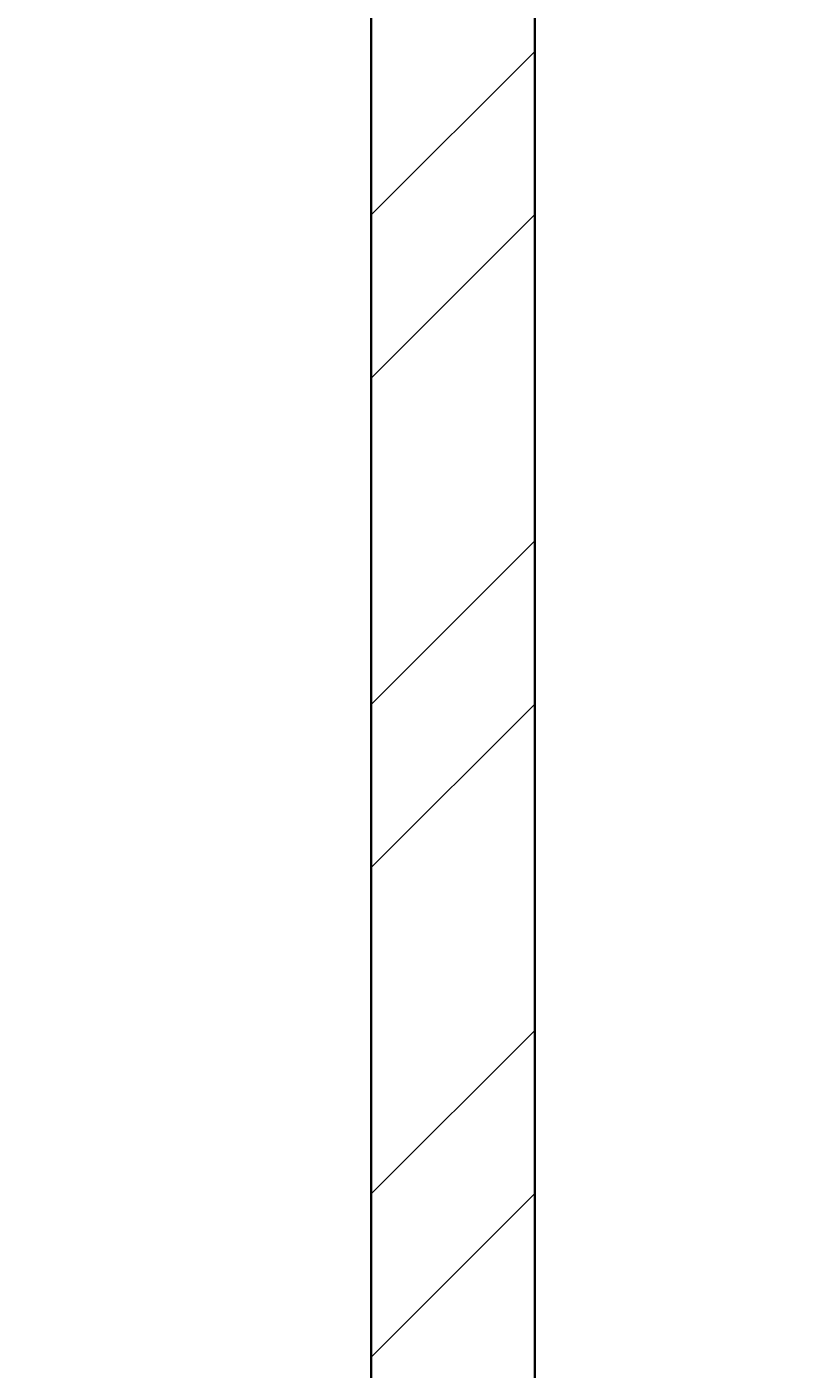
# Model space of a CAD drawing. Units: inches. Extents: x 1962 to 2771, y 1245 to 2660.
# Tile 54 of 114: x 2225 to 2247, y 2068 to 2105. Entities that reach past the tile are written whole.
import ezdxf

# ---------------------------------------------------------------- set-up
doc = ezdxf.new("R2010")
doc.units = ezdxf.units.IN
for name, color, linetype, lineweight in [('A-ANNO-DIMS', 2, 'Continuous', 18), ('A-WALL', 7, 'Continuous', 35), ('A-WALL-PATT', 252, 'Continuous', 13)]:
    doc.layers.add(name, color=color, linetype=linetype, lineweight=lineweight)
doc.styles.get("Standard").update_dxf_attribs({"font": 'arial.ttf'})
doc.dimstyles.get("Standard").update_dxf_attribs({"dimtxt": 0.18, "dimasz": 0.18, "dimexe": 0.18, "dimexo": 0.0625, "dimgap": 0.09, "dimtad": 0, "dimtih": 1, "dimtoh": 1, "dimdec": 4, "dimzin": 0, "dimdsep": 46, "dimtxsty": 'Standard', "dimcen": 0.09, "dimadec": 0, "dimazin": 0, "dimtfac": 1, "dimtdec": 4, "dimtofl": 0, "dimtmove": 0, "dimatfit": 3, "dimfxl": 1, "dimtolj": 1, "dimtzin": 0, "dimarcsym": 0})

# ---------------------------------------------------------------- blocks, each defined once
blk = doc.blocks.new('*D40')
at = {"layer": 'A-ANNO-DIMS', "color": 0, "lineweight": -2, "transparency": 16777216}
for p, q in [((2072.02, 2033.906), (2072.02, 2583.474)), ((2072.2, 2583.294), (2366.02, 2583.294)), ((2660.627, 2583.294), (2366.808, 2583.294)), ((2660.807, 2524.406), (2660.807, 2583.474))]:
    blk.add_line(p, q, dxfattribs=at)
at = {"layer": 'A-ANNO-DIMS', "color": 0, "transparency": 16777216}
for points in [[(2072.2, 2583.324), (2072.2, 2583.264), (2072.02, 2583.294)], [(2660.627, 2583.324), (2660.627, 2583.264), (2660.807, 2583.294)]]:
    blk.add_solid(points, dxfattribs=at)
at = {"layer": 'Defpoints', "color": 0, "transparency": 16777216}
for p in [(2660.807, 2583.294), (2660.807, 2524.344), (2072.02, 2033.844)]:
    blk.add_point(p, dxfattribs=at)
at = {"layer": 'A-ANNO-DIMS', "color": 0, "transparency": 16777216, "insert": (2366.414, 2583.294), "char_height": 0.18, "attachment_point": 5}
blk.add_mtext('\\A1;588.8', dxfattribs=at)

msp = doc.modelspace()

# ---------------------------------------------------------------- hatches: boundary and pattern name
at = {"layer": 'A-WALL-PATT'}
h = msp.add_hatch(dxfattribs=at)
h.set_pattern_fill('ANSI32', color=256)
h.paths.add_polyline_path([(2090.8074, 2467.3437), (2141.6481, 2467.3437), (2141.6481, 2469.5937), (2141.6481, 2471.8437), (2086.3074, 2471.8437), (2086.3074, 2422.5333), (2090.8074, 2422.5333)])
h.paths.add_polyline_path([(2282.7664, 2471.8437), (2204.8982, 2471.8437), (2204.8982, 2467.3437), (2234.8074, 2467.3437), (2234.8074, 2311.3437), (2228.7492, 2311.3437), (2228.7492, 2306.8437), (2234.8074, 2306.8437), (2331.9227, 2306.8437), (2331.9227, 2309.0937), (2331.9227, 2311.3437), (2239.3074, 2311.3437), (2239.3074, 2467.3437), (2282.7664, 2467.3437), (2282.7664, 2469.5937)])
h.paths.add_polyline_path([(2471.4531, 2519.8437), (2552.011, 2519.8437), (2564.3996, 2519.8437), (2564.3996, 2511.1389), (2568.8996, 2511.1389), (2568.8996, 2524.3437), (2466.9531, 2524.3437), (2466.9531, 2471.8437), (2450.0749, 2471.8437), (2446.4672, 2471.8437), (2446.4672, 2467.3437), (2450.0749, 2467.3437), (2475.9988, 2467.3437), (2475.9988, 2469.5937), (2475.9988, 2471.8437), (2471.4531, 2471.8437)])
h.paths.add_polyline_path([(2575.2231, 2469.5937), (2575.2231, 2471.8437), (2568.8996, 2471.8437), (2568.8996, 2487.1389), (2564.3996, 2487.1389), (2564.3996, 2471.8437), (2556.511, 2471.8437), (2499.2904, 2471.8437), (2499.2904, 2467.3437), (2507.8074, 2467.3437), (2507.8074, 2311.3437), (2414.863, 2311.3437), (2414.863, 2306.8437), (2512.3074, 2306.8437), (2517.0114, 2306.8437), (2517.0114, 2309.0937), (2517.0114, 2311.3437), (2512.3074, 2311.3437), (2512.3074, 2467.3437), (2575.2231, 2467.3437)])
h.paths.add_polyline_path([(2660.8074, 2471.8437), (2600.9602, 2471.8437), (2600.9602, 2467.3437), (2656.3074, 2467.3437), (2656.3074, 2432.5704), (2660.8074, 2432.5704)])
h.paths.add_polyline_path([(2660.8074, 2372.5704), (2656.3074, 2372.5704), (2656.3074, 2311.3437), (2600.276, 2311.3437), (2600.276, 2309.0937), (2600.276, 2306.8437), (2656.3074, 2306.8437), (2656.3074, 2296.2593), (2660.8074, 2296.2593)])
h.paths.add_polyline_path([(2572.3074, 2306.8437), (2577.1385, 2306.8437), (2577.1385, 2311.3437), (2551.082, 2311.3437), (2551.082, 2306.8437), (2567.8074, 2306.8437), (2567.8074, 2258.8437), (2540.0574, 2258.8437), (2540.0574, 2256.5937), (2540.0574, 2254.3437), (2567.8074, 2254.3437), (2656.3074, 2254.3437), (2656.3074, 2236.9085), (2660.8074, 2236.9085), (2660.8074, 2272.2593), (2656.3074, 2272.2593), (2656.3074, 2258.8437), (2572.3074, 2258.8437)])
h.paths.add_polyline_path([(2512.3074, 2254.3437), (2518.8716, 2254.3437), (2518.8716, 2256.5937), (2518.8716, 2258.8437), (2507.8074, 2258.8437), (2507.8074, 2177.8437), (2567.8074, 2177.8437), (2567.8074, 2172.9628), (2572.3074, 2172.9628), (2572.3074, 2177.8437), (2656.3074, 2177.8437), (2656.3074, 2166.4846), (2660.8074, 2166.4846), (2660.8074, 2200.9085), (2656.3074, 2200.9085), (2656.3074, 2182.3437), (2512.3074, 2182.3437)])
h.paths.add_polyline_path([(2656.3074, 2129.8437), (2572.3074, 2129.8437), (2572.3074, 2150.3044), (2570.0574, 2150.3044), (2567.8074, 2150.3044), (2567.8074, 2129.8437), (2507.8074, 2129.8437), (2507.8074, 2116.3027), (2510.0574, 2116.3027), (2512.3074, 2116.3027), (2512.3074, 2125.3437), (2567.8074, 2125.3437), (2572.3074, 2125.3437), (2656.3074, 2125.3437)])
h.paths.add_polyline_path([(2090.8074, 2362.5333), (2086.3074, 2362.5333), (2086.3074, 2298.6242), (2090.8074, 2298.6242), (2090.8074, 2306.8437), (2174.8074, 2306.8437), (2174.8074, 2286.4178), (2179.3074, 2286.4178), (2179.3074, 2306.8437), (2192.8641, 2306.8437), (2192.8641, 2309.0937), (2192.8641, 2311.3437), (2090.8074, 2311.3437)])
h.paths.add_polyline_path([(2209.156, 2258.8437), (2179.3074, 2258.8437), (2179.3074, 2263.2236), (2177.0574, 2263.2236), (2174.8074, 2263.2236), (2174.8074, 2258.8437), (2090.8074, 2258.8437), (2090.8074, 2274.6242), (2086.3074, 2274.6242), (2086.3074, 2238.2967), (2088.5574, 2238.2967), (2090.8074, 2238.2967), (2090.8074, 2254.3437), (2209.156, 2254.3437)])
h.paths.add_polyline_path([(2090.8074, 2177.8437), (2234.8074, 2177.8437), (2234.8074, 2173.1428), (2239.3074, 2173.1428), (2239.3074, 2258.8437), (2230.8442, 2258.8437), (2230.8442, 2256.5937), (2230.8442, 2254.3437), (2234.8074, 2254.3437), (2234.8074, 2182.3437), (2090.8074, 2182.3437), (2090.8074, 2202.2967), (2086.3074, 2202.2967), (2086.3074, 2140.0389), (2090.8074, 2140.0389)])
h.paths.add_polyline_path([(2090.8074, 2080.0389), (2086.3074, 2080.0389), (2086.3074, 2033.8437), (2090.8074, 2033.8437)], flags=17)
h.paths.add_polyline_path([(2244.9405, 2033.8437), (2239.3074, 2033.8437), (2239.3074, 2142.0665), (2237.2592, 2142.0665), (2234.8074, 2142.0665), (2234.8074, 2033.8437), (2090.8074, 2033.8437), (2076.5204, 2033.8437), (2072.0204, 2033.8437), (2072.0204, 2000.4493), (2076.5204, 2000.4493), (2076.5204, 2029.3437), (2090.8074, 2029.3437), (2244.9405, 2029.3437), (2244.9405, 2031.5937)])
h.paths.add_polyline_path([(2234.8074, 1933.3437), (2076.5204, 1933.3437), (2076.5204, 1952.4493), (2074.2704, 1952.4493), (2072.0204, 1952.4493), (2072.0204, 1933.3437), (2072.0204, 1928.8437), (2234.8074, 1928.8437)])
h.paths.add_polyline_path([(2090.8074, 1928.8437), (2086.3074, 1928.8437), (2086.3074, 1906.5013), (2090.8074, 1906.5013)])
h.paths.add_polyline_path([(2090.8074, 1846.5013), (2086.3074, 1846.5013), (2086.3074, 1769.9917), (2088.5574, 1769.9917), (2090.8074, 1769.9917), (2090.8074, 1780.3437), (2234.8074, 1780.3437), (2234.8074, 1708.3437), (2230.3764, 1708.3437), (2230.3764, 1703.8437), (2239.3074, 1703.8437), (2239.3074, 1792.6669), (2237.0574, 1792.6669), (2234.8074, 1792.6669), (2234.8074, 1784.8437), (2090.8074, 1784.8437)])
h.paths.add_polyline_path([(2239.3074, 1928.8437), (2244.9405, 1928.8437), (2244.9405, 1931.0937), (2244.9405, 1933.3437), (2234.8074, 1933.3437), (2234.8074, 1928.8437), (2234.8074, 1825.5949), (2239.3074, 1825.5949)])
h.paths.add_polyline_path([(2148.0425, 1649.0937), (2148.0425, 1651.3437), (2090.8074, 1651.3437), (2090.8074, 1646.8437), (2148.0425, 1646.8437)], flags=0)
h.paths.add_polyline_path([(2207.5601, 1708.3437), (2090.8074, 1708.3437), (2090.8074, 1703.8437), (2174.8074, 1703.8437), (2174.8074, 1651.3437), (2170.4457, 1651.3437), (2170.4457, 1646.8437), (2195.9924, 1646.8437), (2195.9924, 1649.0937), (2195.9924, 1651.3437), (2179.3074, 1651.3437), (2179.3074, 1703.8437), (2207.5601, 1703.8437), (2207.5601, 1706.0937)])
h.paths.add_polyline_path([(2090.8074, 1733.9917), (2086.3074, 1733.9917), (2086.3074, 1696.1032), (2088.5574, 1696.1032), (2090.8074, 1696.1032)])
h.paths.add_polyline_path([(2090.8074, 1672.1032), (2086.3074, 1672.1032), (2086.3074, 1600.3335), (2090.8074, 1600.3335)])
h.paths.add_polyline_path([(2090.8074, 1540.3335), (2086.3074, 1540.3335), (2086.3074, 1486.3437), (2139.6766, 1486.3437), (2139.6766, 1490.8437), (2090.8074, 1490.8437)])
h.paths.add_polyline_path([(2302.3876, 1490.8437), (2239.3074, 1490.8437), (2239.3074, 1646.8437), (2335.9994, 1646.8437), (2335.9994, 1651.3437), (2229.884, 1651.3437), (2229.884, 1646.8437), (2234.8074, 1646.8437), (2234.8074, 1490.8437), (2202.7103, 1490.8437), (2202.7103, 1488.5937), (2202.7103, 1486.3437), (2275.0699, 1486.3437), (2275.0699, 1475.772), (2279.5699, 1475.772), (2279.5699, 1486.3437), (2302.3876, 1486.3437)])
h.paths.add_polyline_path([(2279.5699, 1451.772), (2275.0699, 1451.772), (2275.0699, 1438.3437), (2174.8074, 1438.3437), (2174.8074, 1486.3437), (2179.7922, 1486.3437), (2179.7922, 1490.8437), (2163.3585, 1490.8437), (2163.3585, 1488.5937), (2163.3585, 1486.3437), (2170.3074, 1486.3437), (2170.3074, 1433.8437), (2279.5699, 1433.8437)])
h.paths.add_polyline_path([(2427.2363, 1490.8437), (2375.8074, 1490.8437), (2375.8074, 1646.8437), (2381.6401, 1646.8437), (2381.6401, 1651.3437), (2365.887, 1651.3437), (2365.887, 1649.0937), (2365.887, 1646.8437), (2371.3074, 1646.8437), (2371.3074, 1490.8437), (2327.5627, 1490.8437), (2327.5627, 1488.5937), (2327.5627, 1486.3437), (2371.3074, 1486.3437), (2371.3074, 1433.8437), (2375.8074, 1433.8437), (2375.8074, 1486.3437), (2427.2363, 1486.3437)])
h.paths.add_polyline_path([(2512.3074, 1646.8437), (2519.4351, 1646.8437), (2519.4351, 1649.0937), (2519.4351, 1651.3437), (2507.8074, 1651.3437), (2416.0063, 1651.3437), (2416.0063, 1649.0937), (2416.0063, 1646.8437), (2507.8074, 1646.8437), (2507.8074, 1490.8437), (2497.0532, 1490.8437), (2497.0532, 1488.5937), (2497.0532, 1486.3437), (2574.9344, 1486.3437), (2574.9344, 1476.0181), (2579.4344, 1476.0181), (2579.4344, 1486.3437), (2584.4872, 1486.3437), (2584.3074, 1490.8437), (2512.3074, 1490.8437)])
h.paths.add_polyline_path([(2470.5091, 1486.3437), (2473.9767, 1486.3437), (2473.9767, 1490.8437), (2449.6605, 1490.8437), (2449.6605, 1488.5937), (2449.6605, 1486.3437), (2466.0091, 1486.3437), (2466.0091, 1433.8437), (2470.5091, 1433.8437), (2579.4344, 1433.8437), (2579.4344, 1452.0181), (2574.9344, 1452.0181), (2574.9344, 1438.3437), (2554.5091, 1438.3437), (2470.5091, 1438.3437)])
h.paths.add_polyline_path([(2656.3074, 1490.8437), (2611.86, 1490.8437), (2611.86, 1486.3437), (2656.3074, 1486.3437)])
h.paths.add_polyline_path([(2660.8074, 1532.7007), (2658.5574, 1532.7007), (2656.3074, 1532.7007), (2656.3074, 1486.3437), (2660.8074, 1486.3437)])
h.paths.add_polyline_path([(2660.8074, 1664.9663), (2656.3074, 1664.9663), (2656.3074, 1651.3437), (2602.2313, 1651.3437), (2602.2313, 1646.8437), (2656.3074, 1646.8437), (2656.3074, 1592.7007), (2660.8074, 1592.7007)])
h.paths.add_polyline_path([(2660.8074, 1724.5221), (2656.3074, 1724.5221), (2656.3074, 1703.8437), (2542.4725, 1703.8437), (2542.4725, 1699.3437), (2567.8074, 1699.3437), (2567.8074, 1651.3437), (2552.7766, 1651.3437), (2552.7766, 1649.0937), (2552.7766, 1646.8437), (2577.2878, 1646.8437), (2577.2878, 1649.0937), (2577.2878, 1651.3437), (2572.3074, 1651.3437), (2572.3074, 1699.3437), (2656.3074, 1699.3437), (2656.3074, 1688.9663), (2660.8074, 1688.9663)])
h.paths.add_polyline_path([(2660.8074, 1880.6524), (2656.3074, 1880.6524), (2656.3074, 1832.8437), (2512.3074, 1832.8437), (2512.3074, 1837.8959), (2507.8074, 1837.8959), (2507.8074, 1828.3437), (2567.8074, 1828.3437), (2567.8074, 1804.3437), (2572.3074, 1804.3437), (2572.3074, 1828.3437), (2656.3074, 1828.3437), (2656.3074, 1818.6778), (2660.8074, 1818.6778)])
h.paths.add_polyline_path([(2660.8074, 1794.6778), (2656.3074, 1794.6778), (2656.3074, 1780.3437), (2572.3074, 1780.3437), (2572.3074, 1783.0303), (2570.0574, 1783.0303), (2567.8074, 1783.0303), (2567.8074, 1780.3437), (2507.8074, 1780.3437), (2507.8074, 1699.3437), (2517.8858, 1699.3437), (2517.8858, 1701.5937), (2517.8858, 1703.8437), (2512.3074, 1703.8437), (2512.3074, 1775.8437), (2656.3074, 1775.8437), (2656.3074, 1760.5221), (2660.8074, 1760.5221)])
h.paths.add_polyline_path([(2660.8074, 1981.3437), (2660.8074, 2020.2808), (2658.5574, 2020.2808), (2656.3074, 2020.2808), (2656.3074, 1981.3437), (2512.3074, 1981.3437), (2512.3074, 2086.6996), (2507.8074, 2086.6996), (2507.8074, 1981.3437), (2375.8074, 1981.3437), (2375.8074, 1986.8505), (2373.5574, 1986.8505), (2371.3074, 1986.8505), (2371.3074, 1973.2607), (2375.8074, 1973.2607), (2375.8074, 1976.8437), (2507.8074, 1976.8437), (2507.8074, 1865.4281), (2510.0574, 1865.4281), (2512.3074, 1865.4281), (2512.3074, 1976.8437), (2660.8074, 1976.8437)])
h.paths.add_polyline_path([(2375.8074, 1940.297), (2373.5574, 1940.297), (2371.3074, 1940.297), (2371.3074, 1933.3437), (2278.4434, 1933.3437), (2278.4434, 1928.8437), (2371.3074, 1928.8437), (2371.3074, 1651.3437), (2375.8074, 1651.3437)])
h.paths.add_polyline_path([(2660.8074, 1976.8437), (2656.3074, 1976.8437), (2656.3074, 1940.6524), (2660.8074, 1940.6524)], flags=17)
h.paths.add_polyline_path([(2660.8074, 2142.4846), (2656.3074, 2142.4846), (2656.3074, 2080.2808), (2660.8074, 2080.2808)])
h.paths.add_polyline_path([(2381.4189, 2311.3437), (2375.8074, 2311.3437), (2375.8074, 2467.3437), (2424.7242, 2467.3437), (2424.7242, 2469.5937), (2424.7242, 2471.8437), (2375.8074, 2471.8437), (2375.8074, 2524.3437), (2371.3074, 2524.3437), (2371.3074, 2471.8437), (2307.2097, 2471.8437), (2307.2097, 2467.3437), (2371.3074, 2467.3437), (2371.3074, 2311.3437), (2366.8901, 2311.3437), (2366.8901, 2306.8437), (2371.3074, 2306.8437), (2371.3074, 2033.8437), (2279.6589, 2033.8437), (2279.6589, 2029.3437), (2371.3074, 2029.3437), (2371.3074, 2014.2598), (2375.8074, 2014.2598), (2375.8074, 2306.8437), (2381.4189, 2306.8437)])
h.paths.add_polyline_path([(2263.3074, 2524.3437), (2170.3074, 2524.3437), (2170.3074, 2519.8437), (2170.3074, 2471.8437), (2165.0312, 2471.8437), (2165.0312, 2467.3437), (2179.6721, 2467.3437), (2179.6721, 2469.5161), (2179.6721, 2471.8437), (2174.8074, 2471.8437), (2174.8074, 2519.8437), (2258.8074, 2519.8437), (2258.8074, 2511.6436), (2263.3074, 2511.6436)])
h.paths.add_polyline_path([(2245.0232, 1361.4123), (2492.9468, 1361.4123), (2492.9468, 1398.505), (2245.0232, 1398.505)], flags=9)
h.paths.add_polyline_path([(2388.1434, 2086.6936), (2425.0704, 2086.6936), (2425.0704, 2105.3509), (2388.1434, 2105.3509)], flags=9)
h.paths.add_polyline_path([(2404.922, 2242.6744), (2445.7337, 2242.6744), (2445.7337, 2261.3318), (2404.922, 2261.3318)], flags=9)
h.paths.add_polyline_path([(2269.4107, 2156.7935), (2306.3378, 2156.7935), (2306.3378, 2175.4508), (2269.4107, 2175.4508)], flags=9)
h.paths.add_polyline_path([(2269.3277, 2233.4343), (2306.2547, 2233.4343), (2306.2547, 2252.0917), (2269.3277, 2252.0917)], flags=9)
h.paths.add_polyline_path([(2431.6052, 2320.6922), (2470.4456, 2320.6922), (2470.4456, 2339.3495), (2431.6052, 2339.3495)], flags=25)
h.paths.add_polyline_path([(2249.6902, 2315.7608), (2288.5306, 2315.7608), (2288.5306, 2334.4182), (2249.6902, 2334.4182)], flags=25)
h.paths.add_polyline_path([(2096.9301, 2314.3181), (2135.7704, 2314.3181), (2135.7704, 2332.9755), (2096.9301, 2332.9755)], flags=25)
h.paths.add_polyline_path([(2134.3475, 2285.7089), (2161.4655, 2285.7089), (2161.4655, 2304.3662), (2134.3475, 2304.3662)], flags=9)
h.paths.add_polyline_path([(2126.5155, 2209.4076), (2159.9227, 2209.4076), (2159.9227, 2228.065), (2126.5155, 2228.065)], flags=25)
h.paths.add_polyline_path([(2110.5753, 2141.5299), (2149.4157, 2141.5299), (2149.4157, 2160.1872), (2110.5753, 2160.1872)], flags=25)
h.paths.add_polyline_path([(2249.8618, 1968.3317), (2286.3966, 1968.3317), (2286.3966, 1986.989), (2249.8618, 1986.989)], flags=9)
h.paths.add_polyline_path([(2395.9507, 1777.0051), (2436.7624, 1777.0051), (2436.7624, 1795.6625), (2395.9507, 1795.6625)], flags=9)
h.paths.add_polyline_path([(2398.5259, 1888.5651), (2435.0062, 1888.5651), (2435.0062, 1907.2224), (2398.5259, 1907.2224)], flags=25)
h.paths.add_polyline_path([(2259.3506, 1728.3559), (2296.2776, 1728.3559), (2296.2776, 1747.0132), (2259.3506, 1747.0132)], flags=9)
h.paths.add_polyline_path([(2271.3698, 1845.268), (2308.2968, 1845.268), (2308.2968, 1863.9253), (2271.3698, 1863.9253)], flags=9)
h.paths.add_polyline_path([(2120.9355, 1786.3027), (2159.7759, 1786.3027), (2159.7759, 1804.9601), (2120.9355, 1804.9601)], flags=25)
h.paths.add_polyline_path([(2121.3164, 1732.1043), (2154.7236, 1732.1043), (2154.7236, 1750.7616), (2121.3164, 1750.7616)], flags=25)
h.paths.add_polyline_path([(2118.3706, 1678.8997), (2147.5282, 1678.8997), (2147.5282, 1697.557), (2118.3706, 1697.557)], flags=25)
h.paths.add_polyline_path([(2385.9227, 1493.557), (2424.763, 1493.557), (2424.763, 1512.2143), (2385.9227, 1512.2143)], flags=25)
h.paths.add_polyline_path([(2248.7058, 1500.0256), (2287.5462, 1500.0256), (2287.5462, 1518.6829), (2248.7058, 1518.6829)], flags=25)
h.paths.add_polyline_path([(2104.1669, 1617.3771), (2143.0073, 1617.3771), (2143.0073, 1636.0344), (2104.1669, 1636.0344)], flags=9)
h.paths.add_polyline_path([(2096.0714, 1447.8824), (2137.3845, 1447.8824), (2137.3845, 1458.1859), (2096.0714, 1458.1859)], flags=9)
h.paths.add_polyline_path([(2180.6114, 1440.325), (2209.7689, 1440.325), (2209.7689, 1458.9823), (2180.6114, 1458.9823)], flags=25)
h.paths.add_polyline_path([(2316.1698, 1447.9637), (2357.4829, 1447.9637), (2357.4829, 1458.2673), (2316.1698, 1458.2673)], flags=9)
h.paths.add_polyline_path([(2397.6187, 1447.9637), (2438.9318, 1447.9637), (2438.9318, 1458.2673), (2397.6187, 1458.2673)], flags=9)
h.paths.add_polyline_path([(2473.0778, 1439.5953), (2502.2354, 1439.5953), (2502.2354, 1458.2527), (2473.0778, 1458.2527)], flags=25)
h.paths.add_polyline_path([(2589.7027, 1447.8819), (2631.0158, 1447.8819), (2631.0158, 1458.1855), (2589.7027, 1458.1855)], flags=9)
h.paths.add_polyline_path([(2522.4009, 1497.5285), (2561.2413, 1497.5285), (2561.2413, 1516.1859), (2522.4009, 1516.1859)], flags=25)
h.paths.add_polyline_path([(2579.6565, 1671.3482), (2608.8141, 1671.3482), (2608.8141, 1690.0056), (2579.6565, 1690.0056)], flags=25)
h.paths.add_polyline_path([(2544.7038, 1725.5064), (2578.1111, 1725.5064), (2578.1111, 1744.1637), (2544.7038, 1744.1637)], flags=25)
h.paths.add_polyline_path([(2578.1191, 1807.472), (2607.2766, 1807.472), (2607.2766, 1826.1293), (2578.1191, 1826.1293)], flags=25)
h.paths.add_polyline_path([(2595.0614, 1835.1839), (2633.9018, 1835.1839), (2633.9018, 1853.8413), (2595.0614, 1853.8413)], flags=25)
h.paths.add_polyline_path([(2567.0097, 2097.7035), (2605.8501, 2097.7035), (2605.8501, 2116.3609), (2567.0097, 2116.3609)], flags=9)
h.paths.add_polyline_path([(2586.644, 2134.6454), (2615.8015, 2134.6454), (2615.8015, 2153.3027), (2586.644, 2153.3027)], flags=9)
h.paths.add_polyline_path([(2544.6185, 2212.6783), (2578.0258, 2212.6783), (2578.0258, 2231.3356), (2544.6185, 2231.3356)], flags=25)
h.paths.add_polyline_path([(2577.0273, 2256.9023), (2606.1849, 2256.9023), (2606.1849, 2275.5597), (2577.0273, 2275.5597)], flags=24)
h.paths.add_polyline_path([(2605.2683, 2315.2821), (2644.1087, 2315.2821), (2644.1087, 2333.9395), (2605.2683, 2333.9395)], flags=25)
h.paths.add_polyline_path([(2583.1244, 2496.1815), (2624.4375, 2496.1815), (2624.4375, 2506.4851), (2583.1244, 2506.4851)], flags=9)
h.paths.add_polyline_path([(2474.761, 2497.0823), (2503.9185, 2497.0823), (2503.9185, 2515.7397), (2474.761, 2515.7397)], flags=25)
h.paths.add_polyline_path([(2387.5787, 2494.2563), (2428.902, 2494.2563), (2428.902, 2504.5598), (2387.5787, 2504.5598)], flags=9)
h.paths.add_polyline_path([(2300.1657, 2500.1564), (2341.4788, 2500.1564), (2341.4788, 2510.46), (2300.1657, 2510.46)], flags=25)
h.paths.add_polyline_path([(2176.8589, 2497.5843), (2206.0165, 2497.5843), (2206.0165, 2516.2416), (2176.8589, 2516.2416)], flags=25)
h.paths.add_polyline_path([(2097.4668, 2494.9762), (2138.7799, 2494.9762), (2138.7799, 2505.2798), (2097.4668, 2505.2798)], flags=9)

# ---------------------------------------------------------------- linework, layer by layer
at = {"layer": 'A-WALL'}
for p, q in [((2234.8074, 2143.4621), (2234.8074, 2033.8437)), ((2239.3074, 2142.0665), (2239.3074, 2033.8437))]:
    msp.add_line(p, q, dxfattribs=at)

# ---------------------------------------------------------------- dimensions: what is measured, and where the dimension line sits
at = {"layer": 'A-ANNO-DIMS'}
dim = msp.add_linear_dim(base=(2660.8074, 2583.2937), p1=(2072.0204, 2033.8437), p2=(2660.8074, 2524.3437), dimstyle='Standard', override={"dimdec": 1, "dimlfac": 1, "dimrnd": 0, "dimzin": 0, "dimdsep": 46, "dimlunit": 2}, dxfattribs=at)
dim.commit()
dim.dimension.update_dxf_attribs({"geometry": '*D40', "text_midpoint": (2366.4139, 2583.2937)})

doc.saveas('drawing.dxf')
